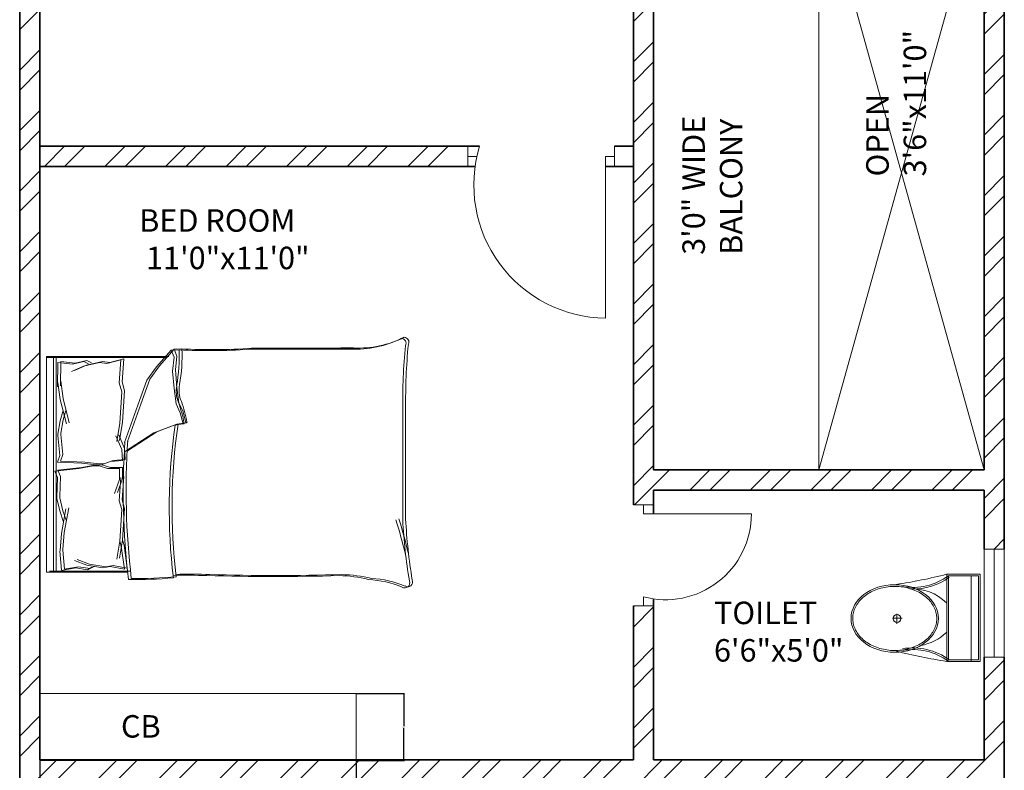
# Model space of a CAD drawing. Units: inches. Extents: x 2168 to 3056, y 1130 to 2629.
# Tile 7 of 42: x 2645 to 2864, y 1789 to 1956. Entities that reach past the tile are written whole.
import ezdxf

# ---------------------------------------------------------------- set-up
doc = ezdxf.new("R2010")
doc.units = ezdxf.units.IN
for name, color, linetype, lineweight in [('A-ANNO-DIMS', 2, 'Continuous', 18), ('A-ANNO-TEXT', 7, 'Continuous', 18), ('A-AREA-IDEN', 7, 'Continuous', 18), ('A-DOOR', 21, 'Continuous', 18), ('A-FLOR-CASE', 71, 'Continuous', 18), ('A-FLOR-FIXT', 9, 'Continuous', 18), ('A-FLOR-OTLN', 7, 'Continuous', 18), ('A-FURN', 8, 'Continuous', 13), ('A-GLAZ', 201, 'Continuous', 18), ('A-WALL', 7, 'Continuous', 35)]:
    doc.layers.add(name, color=color, linetype=linetype, lineweight=lineweight)
doc.layers.add('A-WALL-PATT', color=143, linetype='Continuous', lineweight=13, true_color=0x7aafdf)
doc.styles.get("Standard").update_dxf_attribs({"font": 'arial.ttf'})
doc.dimstyles.get("Standard").update_dxf_attribs({"dimtxt": 0.18, "dimasz": 0.18, "dimexe": 0.18, "dimexo": 0.0625, "dimgap": 0.09, "dimtad": 0, "dimtih": 1, "dimtoh": 1, "dimdec": 4, "dimzin": 0, "dimdsep": 46, "dimtxsty": 'Standard', "dimcen": 0.09, "dimadec": 0, "dimazin": 0, "dimtfac": 1, "dimtdec": 4, "dimtofl": 0, "dimtmove": 0, "dimatfit": 3, "dimfxl": 1, "dimtolj": 1, "dimtzin": 0, "dimarcsym": 0})

# ---------------------------------------------------------------- blocks, each defined once
blk = doc.blocks.new('A$C31115884')
for p, q in [((283.1, 497.7), (223.4, 497.7)), ((257.5, 466.4), (257.5, 523.2)), ((0, 200), (0, 0)), ((520, 200), (0, 200)), ((10, 190), (10, 10)), ((510, 190), (10, 190)), ((510, 10), (510, 190)), ((520, 0), (520, 200)), ((510, 54.5), (0, 54.5)), ((10, 10), (510, 10)), ((0, 0), (520, 0))]:
    blk.add_line(p, q)
blk.add_circle((255.6, 496.4), 23.6)
for centre, radius, start, end in [((2777.7, -204.6), 2807, 165.4549, 171.71327), ((3237, 905), 2807, 188.28673, 194.5451), ((-294.5, 403.3), 364.7, 324.20913, 9.34987), ((-294.5, 403.3), 374.7, 324.20913, 9.34987), ((139.5, 406.2), 293.5, 315.84364, 2.65635), ((805.8, 403.3), 364.7, 170.65013, 215.79087), ((383.6, 406.2), 293.5, 190.27735, 224.15636), ((805.8, 403.3), 374.7, 179.20365, 215.79087)]:
    blk.add_arc(centre, radius, start, end)
blk.add_ellipse((256.2, 509.9), major_axis=(0, -260.7), ratio=0.772727)
blk.add_open_spline([(256.2, 259.2), (263.1, 259.2), (270, 259.7), (287.8, 262.3), (298.7, 265.1), (319.9, 273.1), (330.2, 278.4), (350.1, 291.1), (359.7, 298.7), (377.7, 315.9), (386.2, 325.5), (401.7, 346.6), (408.8, 358.1), (421.3, 382.5), (426.8, 395.5), (435.9, 422.4), (439.5, 436.4), (444.8, 465.1), (446.5, 479.7), (447.9, 509.2), (447.6, 524), (445, 553.3), (442.7, 567.8), (436.3, 596), (432.1, 609.7), (421.9, 636), (416, 648.6), (402.5, 672.1), (395, 683), (378.6, 703), (369.8, 712.1), (351.1, 728), (341.3, 734.8), (320.9, 746.2), (310.4, 750.7), (288.9, 757.3), (278, 759.4), (256, 761), (245, 760.6), (223.1, 757.2), (212.3, 754.3), (191.1, 746.1), (180.8, 740.7), (160.9, 727.8), (151.4, 720.1), (133.5, 702.7), (125.1, 693), (109.6, 671.7), (102.6, 660.2), (90.2, 635.7), (84.9, 622.7), (76, 595.6), (72.4, 581.6), (67.2, 552.9), (65.6, 538.2), (64.4, 508.8), (64.8, 494), (67.5, 464.7), (69.9, 450.2), (76.6, 422), (80.8, 408.3), (91.1, 382.2), (97.2, 369.7), (110.8, 346.3), (118.4, 335.4), (134.8, 315.6), (143.7, 306.7), (162.4, 290.9), (172.3, 284.2), (192.8, 273), (203.3, 268.6), (224.8, 262.2), (235.8, 260.2), (249.9, 259.3), (253, 259.2), (256.2, 259.2)], degree=3, knots=[0, 0, 0, 0, 0.110105, 0.110105, 0.285049, 0.285049, 0.459994, 0.459994, 0.634938, 0.634938, 0.809882, 0.809882, 0.984827, 0.984827, 1.159771, 1.159771, 1.334715, 1.334715, 1.50966, 1.50966, 1.684604, 1.684604, 1.859549, 1.859549, 2.034493, 2.034493, 2.209437, 2.209437, 2.384382, 2.384382, 2.559326, 2.559326, 2.73427, 2.73427, 2.909215, 2.909215, 3.084159, 3.084159, 3.259103, 3.259103, 3.434048, 3.434048, 3.608992, 3.608992, 3.783936, 3.783936, 3.958881, 3.958881, 4.133825, 4.133825, 4.30877, 4.30877, 4.483714, 4.483714, 4.658658, 4.658658, 4.833603, 4.833603, 5.008547, 5.008547, 5.183491, 5.183491, 5.358436, 5.358436, 5.53338, 5.53338, 5.708324, 5.708324, 5.883269, 5.883269, 6.058213, 6.058213, 6.233158, 6.233158, 6.283185, 6.283185, 6.283185, 6.283185])
blk = doc.blocks.new('BED-DOUBLE')
for p, q in [((27.75, 52.87), (24.5, 49.16)), ((27.75, 52.87), (24.5, 49.16)), ((28.39, 53.1), (25.14, 49.39)), ((28.39, 53.1), (25.14, 49.39)), ((29.49, 52.95), (27.75, 52.87, 3.87)), ((29.49, 52.95), (27.75, 52.87, 3.87)), ((28.37, 51.33), (27.75, 52.87)), ((28.37, 51.33), (27.75, 52.87)), ((30.13, 53.18), (28.39, 53.1, 3.87)), ((30.13, 53.18), (28.39, 53.1, 3.87)), ((29, 51.56), (28.39, 53.1)), ((29, 51.56), (28.39, 53.1)), ((0, 51.49), (0.64, 51.49)), ((0, 3.48), (0, 51.49)), ((0, 51.27), (26.61, 51.27)), ((0, 51.27), (26.61, 51.27)), ((0.64, 51.49), (27.25, 51.49)), ((0.64, 51.49), (27.25, 51.49)), ((1.53, 3.48), (1.53, 51.27)), ((1.53, 3.48), (1.53, 51.27)), ((2.17, 3.7), (2.17, 51.49)), ((2.17, 3.7), (2.17, 51.49)), ((6.41, 49.96), (8.98, 50.56)), ((6.41, 49.96), (8.98, 50.56)), ((8.98, 50.56), (10.02, 50.04)), ((8.98, 50.56), (10.02, 50.04)), ((16.57, 50.7), (13.43, 49.92)), ((16.57, 50.7), (13.43, 49.92)), ((17.21, 50.93), (14.07, 50.15)), ((17.21, 50.93), (14.07, 50.15)), ((16.17, 45.57), (16.57, 50.7)), ((16.17, 45.57), (16.57, 50.7)), ((16.81, 45.8), (17.21, 50.93)), ((16.81, 45.79), (17.21, 50.93)), ((28.06, 48.23), (28.37, 51.33)), ((28.06, 48.23), (28.37, 51.33)), ((28.7, 48.46), (29, 51.56)), ((28.7, 48.46), (29, 51.56)), ((2.56, 50.11), (2.46, 44.71)), ((2.56, 50.11), (2.46, 44.71)), ((2.56, 50.11), (5.77, 49.73)), ((2.56, 50.11), (5.77, 49.73)), ((3.2, 50.34), (3.1, 44.94)), ((3.2, 50.34), (3.1, 44.94)), ((3.2, 50.34), (6.41, 49.96)), ((3.2, 50.34), (6.41, 49.96)), ((8.26, 49.31), (5.58, 48.13)), ((8.26, 49.31), (5.58, 48.13)), ((5.77, 49.73), (8.34, 50.33)), ((5.77, 49.73), (8.34, 50.33)), ((8.9, 49.54), (6.22, 48.36)), ((8.9, 49.54), (6.22, 48.36)), ((11.83, 50.11), (8.26, 49.31)), ((11.83, 50.11), (8.26, 49.31)), ((8.34, 50.33), (9.38, 49.81)), ((8.34, 50.33), (9.38, 49.81)), ((12.47, 50.34), (8.9, 49.54)), ((12.47, 50.34), (8.9, 49.54)), ((13.43, 49.92), (11.83, 50.11)), ((13.43, 49.92), (11.83, 50.11)), ((14.07, 50.15), (12.47, 50.34)), ((14.07, 50.15), (12.47, 50.34)), ((24.5, 49.16), (22.33, 46.22)), ((24.5, 49.16), (22.33, 46.22)), ((25.14, 49.39), (22.97, 46.45)), ((25.14, 49.39), (22.97, 46.45)), ((28.37, 44.36), (28.06, 48.23)), ((28.37, 44.36), (28.06, 48.23)), ((29, 44.59), (28.7, 48.46)), ((29, 44.59), (28.7, 48.46)), ((22.33, 46.22), (20.32, 40.64)), ((22.33, 46.22), (20.32, 40.64)), ((22.97, 46.45), (20.96, 40.87)), ((22.97, 46.45), (20.96, 40.87)), ((2.46, 44.71), (2.54, 45.71)), ((2.46, 44.71), (2.54, 45.71)), ((2.54, 45.71), (3.07, 41.91)), ((2.54, 45.71), (3.07, 41.91)), ((3.1, 44.94), (3.18, 45.94)), ((3.1, 44.94), (3.18, 45.94)), ((3.18, 45.94), (3.71, 42.14)), ((3.18, 45.94), (3.71, 42.14)), ((16.73, 43.61), (16.17, 45.57)), ((16.73, 43.61), (16.17, 45.57)), ((17.37, 43.83), (16.81, 45.8)), ((17.37, 43.83), (16.81, 45.79)), ((16.93, 36.82), (17.37, 43.83)), ((16.93, 36.82), (17.37, 43.83)), ((28.83, 40.95), (28.37, 44.36)), ((28.83, 40.95), (28.37, 44.36)), ((29.47, 41.18), (29, 44.59)), ((29.47, 41.18), (29, 44.59)), ((3.07, 41.91), (4.42, 36.5)), ((3.07, 41.91), (4.42, 36.49)), ((3.71, 42.14), (5.06, 36.72)), ((3.71, 42.14), (5.06, 36.72)), ((16.3, 36.6), (16.73, 43.61)), ((16.3, 36.6), (16.73, 43.61)), ((4.31, 39.43), (3.72, 37.36)), ((4.31, 39.43), (3.72, 37.36)), ((20.32, 40.64), (17.38, 32.31)), ((20.32, 40.64), (17.38, 32.31)), ((20.96, 40.87), (18.02, 32.53)), ((20.96, 40.87), (18.02, 32.53)), ((29.76, 38.94), (28.83, 40.95)), ((29.76, 38.94), (28.83, 40.95)), ((30.4, 39.17), (29.47, 41.18)), ((30.4, 39.17), (29.47, 41.18)), ((79.25, 15.06), (79.25, 39.68)), ((79.25, 15.06), (79.25, 39.68)), ((79.88, 15.29), (79.88, 39.91)), ((79.88, 15.29), (79.88, 39.91)), ((3.67, 39.2), (3.08, 37.14)), ((3.67, 39.2), (3.08, 37.14)), ((3.72, 37.36), (3.18, 34.43)), ((3.72, 37.36), (3.18, 34.43)), ((30.38, 36.46), (29.76, 38.94)), ((30.38, 36.46), (29.76, 38.94)), ((31.02, 36.69), (30.4, 39.17)), ((31.02, 36.69), (30.4, 39.17)), ((3.08, 37.14), (2.54, 34.2)), ((3.08, 37.14), (2.54, 34.2)), ((15.63, 32.56), (16.3, 36.6)), ((15.63, 32.56), (16.3, 36.6)), ((16.27, 32.79), (16.93, 36.82)), ((16.27, 32.79), (16.93, 36.82)), ((23.88, 34.45), (28.37, 36.15)), ((23.88, 34.45), (28.37, 36.15)), ((24.52, 34.68), (29, 36.38)), ((24.52, 34.68), (29, 36.38)), ((28.37, 36.15), (30.38, 36.46)), ((28.37, 36.15), (30.38, 36.46)), ((29, 36.38), (31.02, 36.69)), ((29, 36.38), (31.02, 36.69)), ((2.54, 34.2), (2.56, 33.88)), ((2.54, 34.2), (2.56, 33.88)), ((2.56, 33.88), (2.98, 29.46)), ((2.56, 33.88), (2.98, 29.46)), ((3.18, 34.43), (3.2, 34.11)), ((3.18, 34.43), (3.2, 34.11)), ((3.2, 34.11), (3.62, 29.68)), ((3.2, 34.11), (3.62, 29.68)), ((16.74, 30.75), (15.45, 33.82)), ((16.74, 30.75), (15.45, 33.82)), ((17.38, 30.98), (16.09, 34.05)), ((17.38, 30.98), (16.09, 34.05)), ((17.38, 30.26), (23.88, 34.45)), ((17.38, 30.26), (23.88, 34.45)), ((18.02, 30.49), (24.52, 34.68)), ((18.02, 30.49), (24.52, 34.68)), ((16.89, 28.3), (16.74, 30.75)), ((16.89, 28.3), (16.74, 30.75)), ((17.53, 28.53), (17.38, 30.98)), ((17.53, 28.53), (17.38, 30.98)), ((2.98, 29.46), (2.49, 27.98)), ((2.98, 29.46), (2.49, 27.98)), ((3.62, 29.68), (3.13, 28.21)), ((3.62, 29.68), (3.13, 28.21)), ((14.86, 28.36), (17.53, 28.53)), ((14.86, 28.36), (17.53, 28.53)), ((1.87, 25.98), (7.22, 26.56)), ((1.87, 25.98), (7.22, 26.56)), ((2.49, 27.98), (7.87, 27.73)), ((2.49, 27.98), (7.87, 27.73)), ((2.51, 26.21), (7.86, 26.79)), ((2.51, 26.21), (7.86, 26.79)), ((3.13, 28.21), (8.51, 27.96)), ((3.13, 28.21), (8.51, 27.96)), ((7.22, 26.56), (10.4, 27.14)), ((7.22, 26.56), (10.4, 27.14)), ((7.86, 26.79), (11.04, 27.37)), ((7.86, 26.79), (11.04, 27.37)), ((7.87, 27.73), (11.08, 27.36)), ((7.87, 27.73), (11.08, 27.35)), ((8.51, 27.96), (11.72, 27.58)), ((8.51, 27.96), (11.72, 27.58)), ((10.4, 27.14), (11.7, 27.14)), ((10.4, 27.14), (11.7, 27.14)), ((11.04, 27.37), (12.34, 27.37)), ((11.04, 27.37), (12.34, 27.37)), ((11.08, 27.36), (12.38, 27.44)), ((11.08, 27.35), (12.38, 27.44)), ((11.7, 27.14), (13.58, 26.56)), ((11.7, 27.14), (13.58, 26.56)), ((11.72, 27.58), (13.02, 27.66)), ((11.72, 27.58), (13.02, 27.66)), ((12.34, 27.37), (14.22, 26.79)), ((12.34, 27.37), (14.22, 26.79)), ((12.38, 27.44), (14.22, 28.13)), ((12.38, 27.44), (14.22, 28.13)), ((13.02, 27.66), (14.86, 28.36)), ((13.02, 27.66), (14.86, 28.36)), ((13.58, 26.56), (16.26, 26.56)), ((13.58, 26.56), (16.26, 26.56)), ((14.22, 28.13), (16.89, 28.3)), ((14.22, 28.13), (16.89, 28.3)), ((14.22, 26.79), (16.9, 26.79)), ((14.22, 26.79), (16.9, 26.79)), ((16.26, 26.56), (16.26, 24.1)), ((16.26, 26.56), (16.26, 24.1)), ((16.9, 26.79), (16.9, 24.33)), ((16.9, 26.79), (16.9, 24.33)), ((2.45, 24.54), (1.87, 25.98)), ((2.45, 24.54), (1.87, 25.98)), ((2.3, 20.09), (2.45, 24.54)), ((2.3, 20.09), (2.45, 24.54)), ((3.09, 24.77), (2.51, 26.21)), ((3.09, 24.77), (2.51, 26.21)), ((2.94, 20.32), (3.09, 24.77)), ((2.94, 20.32), (3.09, 24.77)), ((16.26, 24.1), (15.17, 20.96)), ((16.26, 24.1), (15.17, 20.96)), ((16.9, 24.33), (15.81, 21.19)), ((16.9, 24.33), (15.81, 21.19)), ((16.17, 19.38), (16.57, 24.52)), ((16.17, 19.38), (16.57, 24.52)), ((16.81, 19.61), (17.21, 24.74)), ((16.81, 19.61), (17.21, 24.74)), ((2.3, 19.77), (2.3, 20.09)), ((2.3, 19.77), (2.3, 20.09)), ((3.03, 16.88), (2.3, 19.77)), ((3.03, 16.88), (2.3, 19.77)), ((2.94, 20), (2.94, 20.32)), ((2.94, 20), (2.94, 20.32)), ((3.67, 17.11), (2.94, 20)), ((3.67, 17.11), (2.94, 20)), ((3.32, 12.11), (4.33, 17.6)), ((3.32, 12.11), (4.33, 17.6)), ((3.96, 12.34), (4.97, 17.83)), ((3.96, 12.34), (4.97, 17.83)), ((16.73, 17.42), (16.17, 19.38)), ((16.73, 17.42), (16.17, 19.38)), ((17.37, 17.65), (16.81, 19.61)), ((17.37, 17.65), (16.81, 19.61)), ((16.93, 10.64), (17.37, 17.65)), ((16.93, 10.64), (17.37, 17.65)), ((3.75, 14.86), (3.03, 16.88)), ((3.75, 14.85), (3.03, 16.88)), ((4.39, 15.08), (3.67, 17.11)), ((4.39, 15.08), (3.67, 17.11)), ((16.3, 10.41), (16.73, 17.42)), ((16.3, 10.41), (16.73, 17.42)), ((3.03, 8.29), (3.32, 12.11)), ((3.03, 8.28), (3.32, 12.11)), ((3.67, 8.51), (3.96, 12.34)), ((3.67, 8.51), (3.96, 12.34)), ((15.63, 6.38), (16.3, 10.41)), ((15.63, 6.38), (16.3, 10.41)), ((16.27, 6.61), (16.93, 10.64)), ((16.27, 6.61), (16.93, 10.64)), ((16.3, 10.41), (16.62, 9.28)), ((16.3, 10.41), (16.62, 9.28)), ((16.62, 9.28), (17.34, 4.18)), ((16.62, 9.28), (17.34, 4.18)), ((16.93, 10.64), (17.26, 9.51)), ((16.93, 10.64), (17.26, 9.51)), ((17.26, 9.51), (17.98, 4.41)), ((17.26, 9.51), (17.98, 4.41)), ((3.01, 8.18), (3.03, 8.29)), ((3.01, 8.18), (3.03, 8.28)), ((3.34, 3.9), (3.01, 8.18)), ((3.34, 3.9), (3.01, 8.18)), ((3.65, 8.41), (3.67, 8.51)), ((3.65, 8.41), (3.67, 8.51)), ((3.98, 4.13), (3.65, 8.41)), ((3.98, 4.13), (3.65, 8.41)), ((3.32, 3.89), (6.5, 4.47)), ((3.32, 3.89), (6.5, 4.47)), ((3.96, 4.12), (7.14, 4.7)), ((3.96, 4.12), (7.14, 4.7)), ((8.96, 5.05), (6.21, 6.06)), ((8.96, 5.05), (6.21, 6.06)), ((6.5, 4.47), (9.1, 4.04)), ((6.5, 4.47), (9.1, 4.04)), ((9.59, 5.28), (6.85, 6.29)), ((9.59, 5.28), (6.85, 6.29)), ((7.14, 4.7), (9.74, 4.27)), ((7.14, 4.7), (9.74, 4.27)), ((12.57, 4.47), (8.96, 5.05)), ((12.57, 4.47), (8.96, 5.05)), ((9.1, 4.04), (10.11, 4.62)), ((9.1, 4.04), (10.11, 4.62)), ((13.21, 4.7), (9.59, 5.28)), ((13.21, 4.7), (9.59, 5.28)), ((9.74, 4.27), (10.75, 4.85)), ((9.74, 4.27), (10.75, 4.85)), ((14.16, 4.76), (12.57, 4.47)), ((14.16, 4.76), (12.57, 4.47)), ((14.8, 4.99), (13.21, 4.7)), ((14.8, 4.99), (13.21, 4.7)), ((17.34, 4.18), (14.16, 4.76)), ((17.34, 4.18), (14.16, 4.76)), ((17.98, 4.41), (14.8, 4.99)), ((17.98, 4.41), (14.8, 4.99)), ((18.11, 3.48), (0, 3.48)), ((18.11, 3.48), (0, 3.48)), ((18.75, 3.7), (0.64, 3.7)), ((18.75, 3.7), (0.64, 3.7))]:
    blk.add_line(p, q)
for centre, radius, start, end in [((68.67, 76.16), 23.07, 267.4714, 296.4681), ((68.67, 76.16), 23.07, 267.4714, 296.4681), ((69.31, 76.39), 23.07, 267.4714, 296.4681), ((69.31, 76.39), 23.07, 267.4714, 296.4681), ((78.87, 54.41), 1.1, 332.6588, 86.02), ((78.87, 54.41), 1.1, 332.6588, 86.02), ((79.51, 54.64), 1.1, 332.6588, 86.02), ((79.51, 54.64), 1.1, 332.6588, 86.02), ((-6.66, 51.33), 36.18, 349.8763, 2.5657), ((-6.66, 51.33), 36.18, 349.8763, 2.5657), ((36.32, 182.27), 129.5, 266.9791, 273.8365), ((36.32, 182.27), 129.5, 266.9791, 273.8365), ((-6.02, 51.56), 36.18, 349.8763, 2.5657), ((-6.02, 51.56), 36.18, 349.8763, 2.5657), ((36.95, 182.49), 129.5, 266.9791, 273.8365), ((36.95, 182.49), 129.5, 266.9791, 273.8365), ((67.82, -4508.74), 4561.86, 90.00217, 90.28689), ((67.82, -4508.74), 4561.86, 90.00217, 90.28689), ((68.46, -4508.51), 4561.86, 90.00217, 90.28689), ((68.46, -4508.52), 4561.86, 90.00217, 90.28689), ((212.28, 41.15), 133.04, 174.4998, 180.6351), ((212.28, 41.15), 133.04, 174.4998, 180.6351), ((212.92, 41.38), 133.04, 174.4998, 180.6351), ((212.92, 41.38), 133.04, 174.4998, 180.6351), ((35.07, 43.74), 6.22, 168.6608, 203.7384), ((35.07, 43.74), 6.22, 168.6608, 203.7384), ((35.71, 43.97), 6.22, 168.6608, 203.7384), ((35.71, 43.97), 6.22, 168.6608, 203.7384), ((1.48, 31.15), 29.65, 10.6617, 19.8806), ((1.48, 31.15), 29.65, 10.6617, 19.8806), ((2.12, 31.38), 29.65, 10.6617, 19.8806), ((2.12, 31.38), 29.65, 10.6617, 19.8806), ((156.32, 17.76), 129.02, 171.7845, 186.9006), ((156.32, 17.76), 129.02, 171.7845, 186.9006), ((156.96, 17.98), 129.02, 171.7845, 186.9006), ((156.96, 17.98), 129.02, 171.7845, 186.9006), ((30.44, 36.64), 0.185, 250.2464, 1.1377), ((30.44, 36.64), 0.185, 250.2464, 1.1377), ((31.08, 36.86), 0.185, 250.2464, 1.1377), ((31.08, 36.86), 0.185, 250.2464, 1.1377), ((182.05, 21.36), 164.97, 176.0865, 186.7821), ((182.05, 21.36), 164.97, 176.0865, 186.7821), ((182.69, 21.59), 164.97, 176.0865, 186.7821), ((182.69, 21.59), 164.97, 176.0865, 186.7821), ((-23.07, -16.99), 106.46, 13.3832, 17.7053), ((-23.07, -16.99), 106.46, 13.3832, 17.7053), ((-23.71, -17.22), 106.46, 13.3832, 17.7053), ((-23.71, -17.22), 106.46, 13.3832, 17.7053), ((200.84, 21.43), 121.76, 182.9958, 189.4091), ((200.84, 21.43), 121.76, 182.9958, 189.4091), ((201.48, 21.66), 121.76, 182.9958, 189.4091), ((201.48, 21.66), 121.76, 182.9958, 189.4091), ((20.1, 85.16), 83.31, 268.7218, 275.604), ((20.1, 85.16), 83.31, 268.7218, 275.604), ((20.74, 85.39), 83.31, 268.7218, 275.604), ((20.74, 85.39), 83.31, 268.7218, 275.604), ((31.17, -167.31), 170.11, 88.4762, 91.0082), ((31.17, -167.31), 170.11, 88.4762, 91.0082), ((31.81, -167.08), 170.11, 88.4762, 91.0082), ((31.81, -167.08), 170.11, 88.4762, 91.0082), ((50.61, 484.82), 482.31, 268.2277, 271.7185), ((50.61, 484.82), 482.31, 268.2277, 271.7185), ((51.25, 485.05), 482.31, 268.2277, 271.7185), ((51.25, 485.05), 482.31, 268.2277, 271.7185), ((64.52, -26.9), 29.63, 76.0648, 88.9113), ((64.52, -26.9), 29.63, 76.0648, 88.9113), ((65.15, -26.67), 29.63, 76.0648, 88.9113), ((65.15, -26.67), 29.63, 76.0648, 88.9113), ((70.28, -21.66), 23.56, 67.9751, 86.652), ((70.28, -21.66), 23.56, 67.9751, 86.652), ((70.92, -21.43), 23.56, 67.9751, 86.652), ((70.92, -21.43), 23.56, 67.9751, 86.652), ((79.72, 1.09), 1.09, 236.1736, 23.4781), ((79.72, 1.09), 1.09, 236.1736, 23.4781), ((80.36, 1.32), 1.09, 236.1736, 23.4781), ((80.36, 1.32), 1.09, 236.1736, 23.4781)]:
    blk.add_arc(centre, radius, start, end)
blk = doc.blocks.new('CUPBOARD-BEDROOM')
blk.add_lwpolyline([(0, 14.89), (70.36, 14.89), (70.36, 0), (0, 0)], close=True)
blk = doc.blocks.new('WIN-24-OPPOSED-JAMBS')
for p, q in [((0, 4.5), (0, 0)), ((0, 4.5), (24, 4.5)), ((24, 2.25), (24, 4.5)), ((24, 4.5), (24, 0)), ((0, 0), (0, 2.25)), ((0, 2.25), (24, 2.25)), ((0, 0), (24, 0))]:
    blk.add_line(p, q)
blk = doc.blocks.new('*D18')
at = {"layer": 'A-ANNO-DIMS', "color": 0, "lineweight": -2, "transparency": 16777216}
for p, q in [((2649.8, 1791.2), (2649.8, 1780.53)), ((2720.15, 1791.2), (2720.15, 1780.53)), ((2649.98, 1780.71), (2683.7, 1780.71)), ((2719.97, 1780.71), (2686.25, 1780.71))]:
    blk.add_line(p, q, dxfattribs=at)
at = {"layer": 'A-ANNO-DIMS', "color": 0, "transparency": 16777216}
for points in [[(2649.98, 1780.74), (2649.98, 1780.68), (2649.8, 1780.71)], [(2719.97, 1780.74), (2719.97, 1780.68), (2720.15, 1780.71)]]:
    blk.add_solid(points, dxfattribs=at)
at = {"layer": 'Defpoints', "color": 0, "transparency": 16777216}
for p in [(2649.8, 1791.27), (2720.15, 1791.27), (2720.15, 1780.71)]:
    blk.add_point(p, dxfattribs=at)
at = {"layer": 'A-ANNO-DIMS', "color": 0, "transparency": 16777216, "insert": (2684.98, 1780.71), "char_height": 0.18, "attachment_point": 5}
blk.add_mtext('\\A1;CUPBOARD 70 TYP.', dxfattribs=at)
blk = doc.blocks.new('*D19')
at = {"layer": 'A-ANNO-DIMS', "color": 0, "lineweight": -2, "transparency": 16777216}
for p, q in [((2720.22, 1806.16), (2730.89, 1806.16)), ((2730.71, 1805.98), (2730.71, 1798.89)), ((2730.71, 1791.45), (2730.71, 1798.53)), ((2720.22, 1791.27), (2730.89, 1791.27))]:
    blk.add_line(p, q, dxfattribs=at)
at = {"layer": 'A-ANNO-DIMS', "color": 0, "transparency": 16777216}
for points in [[(2730.68, 1805.98), (2730.74, 1805.98), (2730.71, 1806.16)], [(2730.68, 1791.45), (2730.74, 1791.45), (2730.71, 1791.27)]]:
    blk.add_solid(points, dxfattribs=at)
at = {"layer": 'Defpoints', "color": 0, "transparency": 16777216}
for p in [(2720.15, 1806.16), (2730.71, 1806.16), (2720.15, 1791.27)]:
    blk.add_point(p, dxfattribs=at)
at = {"layer": 'A-ANNO-DIMS', "color": 0, "transparency": 16777216, "insert": (2730.71, 1798.71), "char_height": 0.18, "attachment_point": 5}
blk.add_mtext('\\A1;15 TYP.', dxfattribs=at)

msp = doc.modelspace()

# ---------------------------------------------------------------- hatches: boundary and pattern name
at = {"layer": 'A-WALL-PATT'}
h = msp.add_hatch(dxfattribs=at)
h.set_pattern_fill('ANSI32', color=256)
h.paths.add_polyline_path([(2463.8, 2409.39), (2467.39, 2409.39), (2467.39, 2413.89), (2454.77, 2413.89), (2454.77, 2411.64), (2454.77, 2409.39), (2459.3, 2409.39), (2459.3, 2265.39), (2455.64, 2265.39), (2455.64, 2260.89), (2467.35, 2260.89), (2467.35, 2263.14), (2467.35, 2265.39), (2463.8, 2265.39)])
h.paths.add_polyline_path([(2431.6, 2413.89), (2409.65, 2413.89), (2409.65, 2409.39), (2431.6, 2409.39), (2431.6, 2411.64)])
h.paths.add_polyline_path([(2349.65, 2413.89), (2331.8, 2413.89), (2331.8, 2362.67), (2336.3, 2362.67), (2336.3, 2409.39), (2349.65, 2409.39), (2349.65, 2411.64)])
h.paths.add_polyline_path([(2634.15, 2411.64), (2634.15, 2413.89), (2562.29, 2413.89), (2562.29, 2409.39), (2595.8, 2409.39), (2595.8, 2280.31), (2595.83, 2280.31), (2595.83, 2265.39), (2499.91, 2265.39), (2499.91, 2260.89), (2550.8, 2260.89), (2550.8, 2117.31), (2555.3, 2117.31), (2555.3, 2168.08), (2571.93, 2168.08), (2571.93, 2176.89), (2559.8, 2176.89), (2559.8, 2256.39), (2640.8, 2256.39), (2640.8, 2176.89), (2626.43, 2176.89), (2626.43, 2168.08), (2645.3, 2168.08), (2645.3, 2116.64), (2649.8, 2116.64), (2649.8, 2260.89), (2691.25, 2260.89), (2691.25, 2263.14), (2691.25, 2265.39), (2670.65, 2265.39), (2670.65, 2265.36), (2600.3, 2265.36), (2600.3, 2280.26), (2600.3, 2409.39), (2634.15, 2409.39)])
h.paths.add_polyline_path([(2600.3, 2473.89), (2612.84, 2473.89), (2612.84, 2478.39), (2572.64, 2478.39), (2572.64, 2473.89), (2595.8, 2473.89), (2595.8, 2413.89), (2600.3, 2413.89)])
h.paths.add_polyline_path([(2535.8, 2473.89), (2548.64, 2473.89), (2548.64, 2478.39), (2531.4, 2478.39), (2531.4, 2413.89), (2521.6, 2413.89), (2521.6, 2409.39), (2539.24, 2409.39), (2539.24, 2411.64), (2539.24, 2413.89), (2535.8, 2413.89)])
h.paths.add_polyline_path([(2664.8, 2478.39), (2636.84, 2478.39), (2636.84, 2473.89), (2660.3, 2473.89), (2660.3, 2413.89), (2656.17, 2413.89), (2656.17, 2409.39), (2671.68, 2409.39), (2671.68, 2411.64), (2671.68, 2413.89), (2664.8, 2413.89)])
h.paths.add_polyline_path([(2705.94, 2413.89), (2695.68, 2413.89), (2695.68, 2409.39), (2705.94, 2409.39)])
h.paths.add_polyline_path([(2741.35, 2413.89), (2728.73, 2413.89), (2728.73, 2411.64), (2728.73, 2409.39), (2732.3, 2409.39), (2732.3, 2265.39), (2725.73, 2265.39), (2725.73, 2260.89), (2740.92, 2260.89), (2740.92, 2263.14), (2740.92, 2265.39), (2736.8, 2265.39), (2736.8, 2409.39), (2741.35, 2409.39)])
h.paths.add_polyline_path([(2785.65, 2413.89), (2764.55, 2413.89), (2764.49, 2409.39), (2785.65, 2409.39), (2785.65, 2411.64)])
h.paths.add_polyline_path([(2864.3, 2413.89), (2845.65, 2413.89), (2845.65, 2409.39), (2859.8, 2409.39), (2859.8, 2368.43), (2864.3, 2368.43)])
h.paths.add_polyline_path([(2864.3, 2308.43), (2862.05, 2308.43), (2859.8, 2308.43), (2859.8, 2265.39), (2774.48, 2265.39), (2774.48, 2263.14), (2774.48, 2260.89), (2781.8, 2260.89), (2781.8, 2226.65), (2786.3, 2226.65), (2786.3, 2260.89), (2859.8, 2260.89), (2859.8, 2241.35), (2864.3, 2241.35)])
h.paths.add_polyline_path([(2864.3, 2217.35), (2862.05, 2217.35), (2859.8, 2217.35), (2859.8, 2200.89), (2786.3, 2200.89), (2786.3, 2205.93), (2784.05, 2205.93), (2781.8, 2205.93), (2781.8, 2150.97), (2786.3, 2150.97), (2786.3, 2161.89), (2859.8, 2161.89), (2859.8, 2144.42), (2864.3, 2144.42)])
h.paths.add_polyline_path([(2859.8, 2196.39), (2859.8, 2166.39), (2786.3, 2166.39), (2786.3, 2196.39)], flags=16)
h.paths.add_polyline_path([(2864.3, 2108.42), (2862.05, 2108.42), (2859.8, 2108.42), (2859.8, 2080.89), (2786.3, 2080.89), (2786.3, 2111.99), (2781.8, 2111.99), (2781.8, 2080.89), (2649.8, 2080.89), (2649.8, 2086.04), (2647.55, 2086.04), (2645.3, 2086.04), (2645.3, 2071.74), (2649.8, 2071.74), (2649.8, 2076.39), (2781.8, 2076.39), (2781.8, 2041.79), (2786.3, 2041.79), (2786.3, 2076.39), (2859.8, 2076.39), (2859.8, 2058.58), (2864.3, 2058.58)])
h.paths.add_polyline_path([(2864.3, 2022.58), (2859.8, 2022.58), (2859.8, 1992.39), (2786.3, 1992.39), (2786.3, 1999.57), (2781.8, 1999.57), (2781.8, 1848.09), (2784.05, 1848.09), (2786.3, 1848.09), (2786.3, 1851.39), (2859.8, 1851.39), (2859.8, 1838.26), (2864.3, 1838.26)], flags=17)
h.paths.add_polyline_path([(2859.8, 1987.89), (2859.8, 1855.89), (2786.3, 1855.89), (2786.3, 1987.89)], flags=16)
h.paths.add_polyline_path([(2823.05, 1987.89), (2841.42, 1921.89), (2823.05, 1855.89)], flags=0)
h.paths.add_polyline_path([(2864.3, 1814.26), (2859.8, 1814.26), (2859.8, 1791.39), (2786.3, 1791.39), (2786.3, 1825.66), (2784.05, 1825.66), (2781.8, 1825.66), (2781.8, 1791.39), (2720.15, 1791.39), (2720.15, 1791.27), (2649.8, 1791.27), (2649.8, 1806.16), (2649.8, 2038.98), (2647.55, 2038.98), (2645.3, 2038.98), (2645.3, 1783.93), (2649.8, 1783.93), (2649.8, 1786.89), (2781.8, 1786.89), (2781.8, 1746.79), (2786.3, 1746.79), (2786.3, 1786.89), (2859.8, 1786.89), (2859.8, 1770.08), (2864.3, 1770.08)])
h.paths.add_polyline_path([(2864.3, 1734.08), (2862.05, 1734.08), (2859.8, 1734.08), (2859.8, 1705.89), (2786.3, 1705.89), (2786.3, 1714.17), (2781.8, 1714.17), (2781.8, 1660.53), (2786.3, 1660.53), (2786.3, 1666.89), (2859.8, 1666.89), (2859.8, 1648.34), (2864.3, 1648.34)])
h.paths.add_polyline_path([(2786.3, 1701.39), (2859.8, 1701.39), (2859.8, 1671.39), (2786.3, 1671.39)], flags=16)
h.paths.add_polyline_path([(2649.8, 1756.58), (2647.55, 1756.58), (2645.3, 1756.58), (2645.3, 1606.89), (2555.3, 1606.89), (2555.3, 1749.51), (2553.05, 1749.51), (2550.8, 1749.51), (2550.8, 1606.89), (2503.01, 1606.89), (2503.01, 1604.64), (2503.01, 1602.39), (2595.8, 1602.39), (2595.85, 1602.39), (2595.85, 1587.5), (2595.8, 1458.39), (2561.5, 1458.39), (2561.5, 1456.14), (2561.5, 1453.89), (2595.8, 1453.89), (2595.8, 1381.89), (2573.44, 1381.89), (2573.44, 1377.39), (2613.01, 1377.39), (2613.01, 1379.64), (2613.01, 1381.89), (2600.3, 1381.89), (2600.3, 1453.89), (2634.33, 1453.89), (2634.33, 1458.39), (2600.3, 1458.39), (2600.3, 1602.39), (2670.65, 1602.39), (2694.09, 1602.39), (2694.09, 1606.89), (2649.8, 1606.89)])
h.paths.add_polyline_path([(2736.8, 1602.39), (2741.56, 1602.39), (2741.56, 1606.89), (2726.2, 1606.89), (2726.2, 1604.64), (2726.2, 1602.39), (2732.3, 1602.39), (2732.3, 1458.39), (2727.9, 1458.39), (2727.9, 1453.89), (2740.82, 1453.89), (2740.82, 1456.14), (2740.82, 1458.39), (2736.8, 1458.39)])
h.paths.add_polyline_path([(2859.8, 1606.89), (2786.3, 1606.89), (2786.3, 1637.33), (2784.05, 1637.33), (2781.8, 1637.33), (2781.8, 1606.89), (2775.61, 1606.89), (2775.61, 1602.39), (2859.8, 1602.39)])
h.paths.add_polyline_path([(2864.3, 1624.34), (2862.05, 1624.34), (2859.8, 1624.34), (2859.8, 1570.39), (2864.3, 1570.39)])
h.paths.add_polyline_path([(2864.3, 1510.39), (2862.05, 1510.39), (2859.8, 1510.39), (2859.8, 1458.39), (2846.73, 1458.39), (2846.73, 1456.14), (2846.73, 1453.89), (2864.3, 1453.89)])
h.paths.add_polyline_path([(2786.73, 1458.39), (2765.44, 1458.39), (2765.44, 1453.89), (2786.73, 1453.89)])
h.paths.add_polyline_path([(2706, 1458.39), (2695.36, 1458.39), (2695.36, 1453.89), (2706, 1453.89), (2706, 1456.14)])
h.paths.add_polyline_path([(2671.36, 1456.14), (2671.36, 1458.39), (2655.99, 1458.39), (2655.99, 1456.14), (2655.99, 1453.89), (2660.3, 1453.89), (2660.3, 1381.89), (2637.01, 1381.89), (2637.01, 1377.39), (2664.8, 1377.39), (2664.8, 1453.89), (2671.36, 1453.89)], flags=17)
h.paths.add_polyline_path([(2539.83, 1458.39), (2520.24, 1458.39), (2520.24, 1453.89), (2531.3, 1453.89), (2531.3, 1377.39), (2546.45, 1377.39), (2546.45, 1379.64), (2546.45, 1381.89), (2535.8, 1381.89), (2535.8, 1453.89), (2539.83, 1453.89)], flags=17)
h.paths.add_polyline_path([(2496.24, 1458.39), (2489.13, 1458.39), (2489.13, 1453.89), (2496.24, 1453.89), (2496.24, 1456.14)])
h.paths.add_polyline_path([(2467.43, 1456.14), (2467.43, 1458.39), (2463.8, 1458.39), (2463.8, 1602.39), (2468.24, 1602.39), (2468.24, 1605.7), (2468.24, 1606.89), (2454.6, 1606.89), (2454.6, 1602.39), (2459.3, 1602.39), (2459.3, 1458.39), (2454.24, 1458.39), (2454.24, 1453.89), (2467.43, 1453.89)])
h.paths.add_polyline_path([(2431.6, 1456.14), (2431.6, 1458.39), (2411.39, 1458.39), (2411.39, 1453.89), (2431.6, 1453.89)])
h.paths.add_polyline_path([(2351.39, 1458.39), (2336.3, 1458.39), (2336.3, 1490.69), (2334.05, 1490.69), (2331.8, 1490.69), (2331.8, 1453.89), (2351.39, 1453.89), (2351.39, 1456.14)])
h.paths.add_polyline_path([(2336.3, 1629.7), (2331.8, 1629.7), (2331.8, 1552.32), (2336.3, 1552.32), (2336.3, 1602.39), (2406.65, 1602.39), (2423.47, 1602.39), (2423.47, 1606.89), (2418.8, 1606.89), (2418.8, 1643.68), (2416.55, 1643.68), (2414.3, 1643.68), (2414.3, 1606.89), (2336.3, 1606.89)])
h.paths.add_polyline_path([(2418.8, 1714.38), (2414.3, 1714.38), (2414.3, 1705.89), (2336.3, 1705.89), (2336.3, 1731.32), (2334.05, 1731.32), (2331.8, 1731.32), (2331.8, 1653.7), (2334.05, 1653.7), (2336.3, 1653.7), (2336.3, 1666.89), (2414.3, 1666.89), (2414.3, 1663.59), (2418.8, 1663.59)])
h.paths.add_polyline_path([(2336.3, 1701.39), (2414.3, 1701.39), (2414.3, 1671.39), (2336.3, 1671.39)], flags=16)
h.paths.add_polyline_path([(2555.3, 2040.06), (2550.8, 2040.06), (2550.8, 1791.39), (2550.56, 1791.2), (2480.2, 1791.2), (2418.8, 1791.39), (2418.8, 1825.45), (2416.55, 1825.45), (2414.3, 1825.45), (2414.3, 1791.39), (2336.3, 1791.39), (2336.3, 1806.41), (2331.8, 1806.41), (2331.8, 1767.32), (2336.3, 1767.32), (2336.3, 1786.89), (2414.3, 1786.89), (2414.3, 1745.46), (2418.8, 1745.46), (2418.8, 1786.89), (2550.8, 1786.89), (2550.8, 1783.01), (2555.3, 1783.01)])
h.paths.add_polyline_path([(2418.8, 1923.39), (2423.21, 1923.39), (2423.21, 1925.64), (2423.21, 1927.89), (2418.8, 1927.89), (2418.8, 2000.05), (2414.3, 2000.05), (2414.3, 1992.39), (2336.3, 1992.39), (2336.3, 1987.89), (2414.3, 1987.89), (2414.3, 1855.89), (2336.3, 1855.89), (2336.3, 1851.39), (2414.3, 1851.39), (2414.3, 1846.76), (2418.8, 1846.76)], flags=17)
h.paths.add_polyline_path([(2336.3, 2019.29), (2334.05, 2019.29), (2331.8, 2019.29), (2331.8, 1830.41), (2336.3, 1830.41)], flags=17)
h.paths.add_polyline_path([(2550.8, 1927.89), (2453.54, 1927.89), (2453.54, 1925.64), (2453.54, 1923.39), (2550.8, 1923.39)], flags=17)
h.paths.add_polyline_path([(2744.99, 1927.89), (2649.8, 1927.89), (2649.8, 1923.39), (2744.99, 1923.39), (2744.99, 1925.64)], flags=17)
h.paths.add_polyline_path([(2555.3, 2086.46), (2553.05, 2086.46), (2550.8, 2086.46), (2550.8, 2080.89), (2418.8, 2080.89), (2336.3, 2080.89), (2336.3, 2115.4), (2334.05, 2115.4), (2331.8, 2115.4), (2331.8, 2055.29), (2336.3, 2055.29), (2336.3, 2076.39), (2550.8, 2076.39), (2550.8, 2071.54), (2555.3, 2071.54)])
h.paths.add_polyline_path([(2418.8, 2121.39), (2414.3, 2121.39), (2414.3, 2080.89), (2418.8, 2080.89)])
h.paths.add_polyline_path([(2418.8, 2076.39), (2414.3, 2076.39), (2414.3, 2035.12), (2418.8, 2035.12)])
h.paths.add_polyline_path([(2422.87, 2263.14), (2422.87, 2265.39), (2406.65, 2265.39), (2406.65, 2265.36), (2336.3, 2265.36), (2336.3, 2280.25), (2336.3, 2302.67), (2334.05, 2302.67), (2331.8, 2302.67), (2331.8, 2246.85), (2336.3, 2246.85), (2336.3, 2260.89), (2414.3, 2260.89), (2414.3, 2224), (2418.8, 2224), (2418.8, 2260.89), (2422.87, 2260.89)])
h.paths.add_polyline_path([(2418.8, 2204.78), (2416.55, 2204.78), (2414.3, 2204.78), (2414.3, 2200.89), (2336.3, 2200.89), (2336.3, 2220.85), (2331.8, 2220.85), (2331.8, 2151.4), (2336.3, 2151.4), (2336.3, 2161.89), (2414.3, 2161.89), (2414.3, 2153.73), (2418.8, 2153.73)])
h.paths.add_polyline_path([(2414.3, 2196.39), (2414.3, 2166.39), (2336.3, 2166.39), (2336.3, 2196.39)], flags=16)
h.paths.add_polyline_path([(2375.3, 2181.39), (2336.3, 2166.39), (2336.3, 2196.39)], flags=0)
h.paths.add_polyline_path([(2809.6, 2172.34), (2838.8, 2172.34), (2838.8, 2191), (2809.6, 2191)], flags=8)
h.paths.add_polyline_path([(2849.75, 1919.59), (2849.75, 1952.67), (2831.09, 1952.67), (2831.09, 1919.59)], flags=8)
h.paths.add_polyline_path([(2808.87, 1901.97), (2808.87, 1937.85), (2790.15, 1937.85), (2790.15, 1901.97)], flags=8)
h.paths.add_polyline_path([(2806.28, 1671.9), (2835.49, 1671.9), (2835.49, 1690.55), (2806.28, 1690.55)], flags=8)
h.paths.add_polyline_path([(2353.19, 1676.55), (2382.39, 1676.55), (2382.39, 1695.21), (2353.19, 1695.21)], flags=8)
h.paths.add_polyline_path([(2360.08, 1832.31), (2389.24, 1832.31), (2389.24, 1850.97), (2360.08, 1850.97)], flags=25)
h.paths.add_polyline_path([(2354.82, 2167.82), (2384.03, 2167.82), (2384.03, 2186.48), (2354.82, 2186.48)], flags=8)

# ---------------------------------------------------------------- linework, layer by layer
at = {"layer": 'A-DOOR'}
for p, q in [((2744.99, 1923.39), (2744.99, 1927.89)), ((2744.99, 1927.89), (2744.99, 1923.39)), ((2777.61, 1927.89), (2777.61, 1923.39)), ((2744.99, 1923.39), (2744.99, 1925.64)), ((2744.99, 1925.64), (2746.99, 1925.64)), ((2777.61, 1925.64), (2775.61, 1925.64)), ((2775.61, 1925.64), (2775.61, 1889.64)), ((2777.61, 1923.39), (2777.61, 1925.64)), ((2786.3, 1848.09), (2781.8, 1848.09)), ((2781.8, 1848.09), (2784.05, 1848.09)), ((2784.05, 1848.09), (2784.05, 1846.09)), ((2784.05, 1846.09), (2808.05, 1846.09)), ((2784.05, 1825.66), (2784.05, 1827.66)), ((2781.8, 1825.66), (2786.3, 1825.66)), ((2786.3, 1825.66), (2784.05, 1825.66))]:
    msp.add_line(p, q, dxfattribs=at)
for centre, radius, start, end in [((2775.97, 1919.31), 29.67, 163.1891, 269.2866), ((2788.97, 1846.09), 19.07, 255.0338, 360)]:
    msp.add_arc(centre, radius, start, end, dxfattribs=at)
at = {"layer": 'A-FLOR-OTLN'}
for p, q in [((2823.05, 1987.89), (2823.05, 1855.89)), ((2823.05, 1855.89), (2859.8, 1987.89)), ((2823.05, 1987.89), (2859.8, 1855.89))]:
    msp.add_line(p, q, dxfattribs=at)
at = {"layer": 'A-WALL'}
for p, q in [((2645.3, 2038.98), (2645.3, 1783.93)), ((2649.8, 1791.39), (2649.8, 2040.56)), ((2864.3, 2022.58), (2864.3, 1838.26)), ((2781.8, 1999.57), (2781.8, 1848.09)), ((2786.3, 1987.89), (2786.3, 1855.89)), ((2859.8, 1987.89), (2859.8, 1855.89)), ((2649.8, 1923.39), (2649.8, 1927.89)), ((2649.8, 1927.89), (2747.57, 1927.89)), ((2777.61, 1927.89), (2781.8, 1927.89)), ((2781.8, 1927.89), (2781.8, 1927.89)), ((2746.59, 1923.39), (2649.8, 1923.39)), ((2781.8, 1923.39), (2775.61, 1923.39)), ((2781.8, 1848.09), (2781.8, 1923.39)), ((2786.3, 1855.89), (2859.8, 1855.89)), ((2786.3, 1851.39), (2859.8, 1851.39)), ((2786.3, 1851.39), (2786.3, 1846.09)), ((2859.8, 1851.39), (2859.8, 1838.26)), ((2786.3, 1827.2), (2786.3, 1791.39)), ((2781.8, 1791.39), (2781.8, 1825.66)), ((2781.8, 1825.66), (2781.8, 1791.39)), ((2859.8, 1814.26), (2859.8, 1791.39)), ((2864.3, 1814.26), (2864.3, 1648.34)), ((2649.8, 1791.39), (2781.8, 1791.39)), ((2786.3, 1791.39), (2859.8, 1791.39))]:
    msp.add_line(p, q, dxfattribs=at)

# ---------------------------------------------------------------- block references
at = {"layer": 'A-FLOR-CASE'}
msp.add_blockref('CUPBOARD-BEDROOM', (2649.8, 1791.26), dxfattribs=at)
at = {"layer": 'A-FLOR-FIXT', "xscale": 0.0372717239612423, "yscale": 0.0372717239612423, "zscale": 0.0372717239612423, "rotation": 89.99999999999999}
msp.add_blockref('A$C31115884', (2858.93, 1813.31), dxfattribs=at)
at = {"layer": 'A-FURN'}
msp.add_blockref('BED-DOUBLE', (2651.25, 1829.66), dxfattribs=at)
at = {"layer": 'A-GLAZ', "rotation": 270}
msp.add_blockref('WIN-24-OPPOSED-JAMBS', (2859.8, 1838.26), dxfattribs=at)

# ---------------------------------------------------------------- texts
at = {"layer": 'A-ANNO-TEXT', "insert": (2661.71, 1801.35), "char_height": 5, "attachment_point": 1}
msp.add_mtext_dynamic_manual_height_columns('    CB', width=30.0271, gutter_width=12.5, heights=[0], dxfattribs=at)
at = {"layer": 'A-AREA-IDEN', "char_height": 5, "attachment_point": 1, "rotation": 90}
for s, width, insert in [('OPEN\\P3\'6"x11\'0"', 119.8185, (2833.58, 1921.17)), ('3\'0" WIDE\\PBALCONY', 100.0048, (2792.7, 1903.73))]:
    msp.add_mtext_dynamic_manual_height_columns(s, width=width, gutter_width=12.5, heights=[0], dxfattribs=dict(at, insert=insert))
at = {"layer": 'A-AREA-IDEN', "char_height": 5, "attachment_point": 1}
for s, width, insert in [('       BED ROOM\\P        11\'0"x11\'0"', 118.2863, (2661.18, 1913.87)), ('TOILET\\P6\'6"x5\'0"', 95.3243, (2799.72, 1826.59))]:
    msp.add_mtext_dynamic_manual_height_columns(s, width=width, gutter_width=12.5, heights=[0], dxfattribs=dict(at, insert=insert))

# ---------------------------------------------------------------- dimensions: what is measured, and where the dimension line sits
at = {"layer": 'A-ANNO-DIMS'}
dim = msp.add_linear_dim(base=(2730.71, 1806.16), p1=(2720.15, 1791.27), p2=(2720.15, 1806.16), angle=90, text='<> TYP.', dimstyle='Standard', override={"dimdec": 0, "dimlfac": 1, "dimrnd": 0, "dimzin": 0, "dimdsep": 46, "dimlunit": 2}, dxfattribs=at)
dim.commit()
dim.dimension.update_dxf_attribs({"geometry": '*D19', "text_midpoint": (2730.71, 1798.71)})
dim = msp.add_linear_dim(base=(2720.15, 1780.71), p1=(2649.8, 1791.27), p2=(2720.15, 1791.27), text='CUPBOARD <> TYP.', dimstyle='Standard', override={"dimdec": 0, "dimlfac": 1, "dimrnd": 0, "dimzin": 0, "dimdsep": 46, "dimlunit": 2}, dxfattribs=at)
dim.commit()
dim.dimension.update_dxf_attribs({"geometry": '*D18', "text_midpoint": (2684.98, 1780.71)})

doc.saveas('drawing.dxf')
